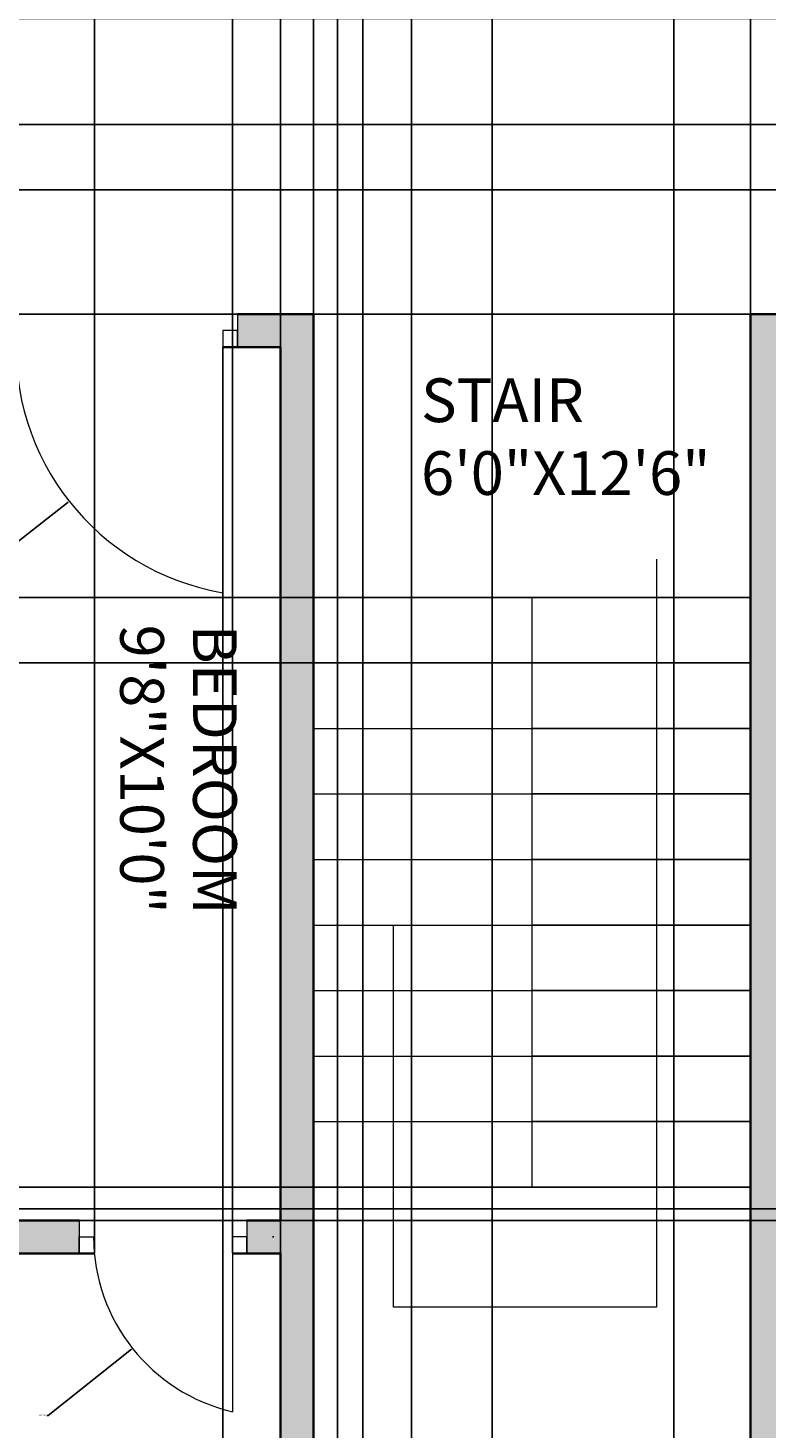
# Model space of a CAD drawing. Units: inches. Extents: x 2606 to 3027, y 1906 to 2463.
# Tile 3 of 10: x 2748 to 2850, y 2004 to 2196. Entities that reach past the tile are written whole.
import ezdxf

# ---------------------------------------------------------------- set-up
doc = ezdxf.new("R2010")
doc.units = ezdxf.units.IN
for name, color, linetype, lineweight in [('A-ANNO-DIMS', 2, 'Continuous', 18), ('A-AREA-IDEN', 7, 'Continuous', 18), ('A-DOOR', 3, 'Continuous', 18), ('A-FLOR-STRS', 7, 'Continuous', 18), ('A-WALL', 7, 'Continuous', 35)]:
    doc.layers.add(name, color=color, linetype=linetype, lineweight=lineweight)
doc.layers.add('A-WALL-PATT', color=251, linetype='Continuous', lineweight=13, true_color=0x636466)
doc.styles.get("Standard").update_dxf_attribs({"font": 'arial.ttf'})
doc.dimstyles.get("Standard").update_dxf_attribs({"dimtxt": 0.18, "dimasz": 0.18, "dimexe": 0.18, "dimexo": 0.0625, "dimgap": 0.09, "dimtad": 0, "dimtih": 1, "dimtoh": 1, "dimdec": 4, "dimzin": 0, "dimdsep": 46, "dimtxsty": 'Standard', "dimcen": 0.09, "dimadec": 0, "dimazin": 0, "dimtfac": 1, "dimtdec": 4, "dimtofl": 0, "dimtmove": 0, "dimatfit": 3, "dimfxl": 1, "dimtolj": 1, "dimtzin": 0, "dimarcsym": 0})

# ---------------------------------------------------------------- blocks, each defined once
blk = doc.blocks.new('*D34')
at = {"layer": 'A-ANNO-DIMS', "color": 0, "lineweight": -2, "transparency": 16777216}
for p, q in [((2787.56, 2118.27), (2787.56, 2433.99)), ((2787.74, 2433.81), (2817.34, 2433.81)), ((2847.38, 2433.81), (2817.78, 2433.81)), ((2847.56, 2118.27), (2847.56, 2433.99))]:
    blk.add_line(p, q, dxfattribs=at)
at = {"layer": 'A-ANNO-DIMS', "color": 0, "transparency": 16777216}
for points in [[(2787.74, 2433.84), (2787.74, 2433.78), (2787.56, 2433.81)], [(2847.38, 2433.84), (2847.38, 2433.78), (2847.56, 2433.81)]]:
    blk.add_solid(points, dxfattribs=at)
at = {"layer": 'Defpoints', "color": 0, "transparency": 16777216}
for p in [(2847.56, 2433.81), (2787.56, 2118.21), (2847.56, 2118.21)]:
    blk.add_point(p, dxfattribs=at)
at = {"layer": 'A-ANNO-DIMS', "color": 0, "transparency": 16777216, "insert": (2817.56, 2433.81), "char_height": 0.18, "attachment_point": 5}
blk.add_mtext('\\A1;60', dxfattribs=at)
blk = doc.blocks.new('*D35')
at = {"layer": 'A-ANNO-DIMS', "color": 0, "lineweight": -2, "transparency": 16777216}
for p, q in [((2801.04, 1993.17), (2801.04, 2433.99)), ((2801.22, 2433.81), (2818.82, 2433.81)), ((2836.86, 2433.81), (2819.26, 2433.81)), ((2837.04, 1993.17), (2837.04, 2433.99))]:
    blk.add_line(p, q, dxfattribs=at)
at = {"layer": 'A-ANNO-DIMS', "color": 0, "transparency": 16777216}
for points in [[(2801.22, 2433.84), (2801.22, 2433.78), (2801.04, 2433.81)], [(2836.86, 2433.84), (2836.86, 2433.78), (2837.04, 2433.81)]]:
    blk.add_solid(points, dxfattribs=at)
at = {"layer": 'Defpoints', "color": 0, "transparency": 16777216}
for p in [(2837.04, 2433.81), (2801.04, 1993.11), (2837.04, 1993.11)]:
    blk.add_point(p, dxfattribs=at)
at = {"layer": 'A-ANNO-DIMS', "color": 0, "transparency": 16777216, "insert": (2819.04, 2433.81), "char_height": 0.18, "attachment_point": 5}
blk.add_mtext('\\A1;36', dxfattribs=at)
blk = doc.blocks.new('*D36')
at = {"layer": 'A-ANNO-DIMS', "color": 0, "lineweight": -2, "transparency": 16777216}
for p, q in [((2787.56, 1993.17), (2787.56, 2433.99)), ((2787.74, 2433.81), (2793.85, 2433.81)), ((2800.86, 2433.81), (2794.76, 2433.81)), ((2801.04, 1993.17), (2801.04, 2433.99))]:
    blk.add_line(p, q, dxfattribs=at)
at = {"layer": 'A-ANNO-DIMS', "color": 0, "transparency": 16777216}
for points in [[(2787.74, 2433.84), (2787.74, 2433.78), (2787.56, 2433.81)], [(2800.86, 2433.84), (2800.86, 2433.78), (2801.04, 2433.81)]]:
    blk.add_solid(points, dxfattribs=at)
at = {"layer": 'Defpoints', "color": 0, "transparency": 16777216}
for p in [(2787.56, 2433.81), (2787.56, 1993.11), (2801.04, 1993.11)]:
    blk.add_point(p, dxfattribs=at)
at = {"layer": 'A-ANNO-DIMS', "color": 0, "transparency": 16777216, "insert": (2794.3, 2433.81), "char_height": 0.18, "attachment_point": 5}
blk.add_mtext('\\A1;13.478', dxfattribs=at)
blk = doc.blocks.new('*D38')
at = {"layer": 'A-ANNO-DIMS', "color": 0, "lineweight": -2, "transparency": 16777216}
for p, q in [((2783.06, 1993.17), (2783.06, 2433.99)), ((2783.24, 2433.81), (2785.05, 2433.81)), ((2787.38, 2433.81), (2785.57, 2433.81)), ((2787.56, 1993.17), (2787.56, 2433.99))]:
    blk.add_line(p, q, dxfattribs=at)
at = {"layer": 'A-ANNO-DIMS', "color": 0, "transparency": 16777216}
for points in [[(2783.24, 2433.84), (2783.24, 2433.78), (2783.06, 2433.81)], [(2787.38, 2433.84), (2787.38, 2433.78), (2787.56, 2433.81)]]:
    blk.add_solid(points, dxfattribs=at)
at = {"layer": 'Defpoints', "color": 0, "transparency": 16777216}
for p in [(2787.56, 2433.81), (2783.06, 1993.11), (2787.56, 1993.11)]:
    blk.add_point(p, dxfattribs=at)
at = {"layer": 'A-ANNO-DIMS', "color": 0, "transparency": 16777216, "insert": (2785.31, 2433.81), "char_height": 0.18, "attachment_point": 5}
blk.add_mtext('\\A1;4.5', dxfattribs=at)
blk = doc.blocks.new('*D39')
at = {"layer": 'A-ANNO-DIMS', "color": 0, "lineweight": -2, "transparency": 16777216}
for p, q in [((2847.5, 2118.21), (2634.68, 2118.21)), ((2634.86, 2118.03), (2634.86, 2113.89)), ((2634.86, 2109.39), (2634.86, 2113.53)), ((2847.5, 2109.21), (2634.68, 2109.21))]:
    blk.add_line(p, q, dxfattribs=at)
at = {"layer": 'A-ANNO-DIMS', "color": 0, "transparency": 16777216}
for points in [[(2634.83, 2118.03), (2634.89, 2118.03), (2634.86, 2118.21)], [(2634.83, 2109.39), (2634.89, 2109.39), (2634.86, 2109.21)]]:
    blk.add_solid(points, dxfattribs=at)
at = {"layer": 'Defpoints', "color": 0, "transparency": 16777216}
for p in [(2847.56, 2118.21), (2634.86, 2109.21), (2847.56, 2109.21)]:
    blk.add_point(p, dxfattribs=at)
at = {"layer": 'A-ANNO-DIMS', "color": 0, "transparency": 16777216, "insert": (2634.86, 2113.71), "char_height": 0.18, "attachment_point": 5}
blk.add_mtext('\\A1;9', dxfattribs=at)
blk = doc.blocks.new('*D40')
at = {"layer": 'A-ANNO-DIMS', "color": 0, "lineweight": -2, "transparency": 16777216}
for p, q in [((2847.5, 2037.21), (2634.68, 2037.21)), ((2634.86, 2037.03), (2634.86, 2015.34)), ((2634.86, 1993.29), (2634.86, 2014.98)), ((2847.5, 1993.11), (2634.68, 1993.11))]:
    blk.add_line(p, q, dxfattribs=at)
at = {"layer": 'A-ANNO-DIMS', "color": 0, "transparency": 16777216}
for points in [[(2634.83, 2037.03), (2634.89, 2037.03), (2634.86, 2037.21)], [(2634.83, 1993.29), (2634.89, 1993.29), (2634.86, 1993.11)]]:
    blk.add_solid(points, dxfattribs=at)
at = {"layer": 'Defpoints', "color": 0, "transparency": 16777216}
for p in [(2847.56, 2037.21), (2634.86, 1993.11), (2847.56, 1993.11)]:
    blk.add_point(p, dxfattribs=at)
at = {"layer": 'A-ANNO-DIMS', "color": 0, "transparency": 16777216, "insert": (2634.86, 2015.16), "char_height": 0.18, "attachment_point": 5}
blk.add_mtext('\\A1;44.1', dxfattribs=at)
blk = doc.blocks.new('*D41')
at = {"layer": 'A-ANNO-DIMS', "color": 0, "lineweight": -2, "transparency": 16777216}
for p, q in [((2787.63, 2157.11), (3000.44, 2157.11)), ((3000.26, 2156.93), (3000.26, 2075.29)), ((3000.26, 1993.29), (3000.26, 2074.93)), ((2787.63, 1993.11), (3000.44, 1993.11))]:
    blk.add_line(p, q, dxfattribs=at)
at = {"layer": 'A-ANNO-DIMS', "color": 0, "transparency": 16777216}
for points in [[(3000.23, 2156.93), (3000.29, 2156.93), (3000.26, 2157.11)], [(3000.23, 1993.29), (3000.29, 1993.29), (3000.26, 1993.11)]]:
    blk.add_solid(points, dxfattribs=at)
at = {"layer": 'Defpoints', "color": 0, "transparency": 16777216}
for p in [(2787.56, 2157.11), (2787.56, 1993.11), (3000.26, 1993.11)]:
    blk.add_point(p, dxfattribs=at)
at = {"layer": 'A-ANNO-DIMS', "color": 0, "transparency": 16777216, "insert": (3000.26, 2075.11), "char_height": 0.18, "attachment_point": 5}
blk.add_mtext('\\A1;164', dxfattribs=at)
blk = doc.blocks.new('*D43')
at = {"layer": 'A-ANNO-DIMS', "color": 0, "lineweight": -2, "transparency": 16777216}
for p, q in [((2794.34, 2257.55), (2794.34, 1965.23)), ((2812.09, 2257.55), (2812.09, 1965.23)), ((2794.52, 1965.41), (2802.76, 1965.41)), ((2811.91, 1965.41), (2803.67, 1965.41))]:
    blk.add_line(p, q, dxfattribs=at)
at = {"layer": 'A-ANNO-DIMS', "color": 0, "transparency": 16777216}
for points in [[(2794.52, 1965.44), (2794.52, 1965.38), (2794.34, 1965.41)], [(2811.91, 1965.44), (2811.91, 1965.38), (2812.09, 1965.41)]]:
    blk.add_solid(points, dxfattribs=at)
at = {"layer": 'Defpoints', "color": 0, "transparency": 16777216}
for p in [(2794.34, 2257.61), (2812.09, 2257.61), (2812.09, 1965.41)]:
    blk.add_point(p, dxfattribs=at)
at = {"layer": 'A-ANNO-DIMS', "color": 0, "transparency": 16777216, "insert": (2803.22, 1965.41), "char_height": 0.18, "attachment_point": 5}
blk.add_mtext('\\A1;17.756', dxfattribs=at)
blk = doc.blocks.new('*D45')
at = {"layer": 'A-ANNO-DIMS', "color": 0, "lineweight": -2, "transparency": 16777216}
for p, q in [((2746.75, 2152.55), (2746.75, 1965.23)), ((2775.13, 2152.55), (2775.13, 1965.23)), ((2746.93, 1965.41), (2760.47, 1965.41)), ((2774.95, 1965.41), (2761.4, 1965.41))]:
    blk.add_line(p, q, dxfattribs=at)
at = {"layer": 'A-ANNO-DIMS', "color": 0, "transparency": 16777216}
for points in [[(2746.93, 1965.44), (2746.93, 1965.38), (2746.75, 1965.41)], [(2774.95, 1965.44), (2774.95, 1965.38), (2775.13, 1965.41)]]:
    blk.add_solid(points, dxfattribs=at)
at = {"layer": 'Defpoints', "color": 0, "transparency": 16777216}
for p in [(2746.75, 2152.61), (2775.13, 2152.61), (2775.13, 1965.41)]:
    blk.add_point(p, dxfattribs=at)
at = {"layer": 'A-ANNO-DIMS', "color": 0, "transparency": 16777216, "insert": (2760.94, 1965.41), "char_height": 0.18, "attachment_point": 5}
blk.add_mtext('\\A1;28.384', dxfattribs=at)
blk = doc.blocks.new('*D47')
at = {"layer": 'A-ANNO-DIMS', "color": 0, "lineweight": -2, "transparency": 16777216}
for p, q in [((2757.51, 2028.17), (2757.51, 2433.99)), ((2757.69, 2433.81), (2766.59, 2433.81)), ((2776.27, 2433.81), (2767.36, 2433.81)), ((2776.45, 2028.17), (2776.45, 2433.99))]:
    blk.add_line(p, q, dxfattribs=at)
at = {"layer": 'A-ANNO-DIMS', "color": 0, "transparency": 16777216}
for points in [[(2757.69, 2433.84), (2757.69, 2433.78), (2757.51, 2433.81)], [(2776.27, 2433.84), (2776.27, 2433.78), (2776.45, 2433.81)]]:
    blk.add_solid(points, dxfattribs=at)
at = {"layer": 'Defpoints', "color": 0, "transparency": 16777216}
for p in [(2776.45, 2433.81), (2757.51, 2028.11), (2776.45, 2028.11)]:
    blk.add_point(p, dxfattribs=at)
at = {"layer": 'A-ANNO-DIMS', "color": 0, "transparency": 16777216, "insert": (2766.98, 2433.81), "char_height": 0.18, "attachment_point": 5}
blk.add_mtext('\\A1;18.94', dxfattribs=at)
blk = doc.blocks.new('*D52')
at = {"layer": 'A-ANNO-DIMS', "color": 0, "lineweight": -2, "transparency": 16777216}
for p, q in [((2787.56, 2257.55), (2787.56, 1965.23)), ((2794.34, 2257.55), (2794.34, 1965.23)), ((2787.74, 1965.41), (2790.56, 1965.41)), ((2794.16, 1965.41), (2791.34, 1965.41))]:
    blk.add_line(p, q, dxfattribs=at)
at = {"layer": 'A-ANNO-DIMS', "color": 0, "transparency": 16777216}
for points in [[(2787.74, 1965.44), (2787.74, 1965.38), (2787.56, 1965.41)], [(2794.16, 1965.44), (2794.16, 1965.38), (2794.34, 1965.41)]]:
    blk.add_solid(points, dxfattribs=at)
at = {"layer": 'Defpoints', "color": 0, "transparency": 16777216}
for p in [(2787.56, 2257.61), (2794.34, 2257.61), (2794.34, 1965.41)]:
    blk.add_point(p, dxfattribs=at)
at = {"layer": 'A-ANNO-DIMS', "color": 0, "transparency": 16777216, "insert": (2790.95, 1965.41), "char_height": 0.18, "attachment_point": 5}
blk.add_mtext('\\A1;6.776', dxfattribs=at)
blk = doc.blocks.new('*D54')
at = {"layer": 'A-ANNO-DIMS', "color": 0, "lineweight": -2, "transparency": 16777216}
for p, q in [((2775.13, 2152.55), (2775.13, 1965.23)), ((2783.06, 2152.55), (2783.06, 1965.23)), ((2775.31, 1965.41), (2778.7, 1965.41)), ((2782.88, 1965.41), (2779.49, 1965.41))]:
    blk.add_line(p, q, dxfattribs=at)
at = {"layer": 'A-ANNO-DIMS', "color": 0, "transparency": 16777216}
for points in [[(2775.31, 1965.44), (2775.31, 1965.38), (2775.13, 1965.41)], [(2782.88, 1965.44), (2782.88, 1965.38), (2783.06, 1965.41)]]:
    blk.add_solid(points, dxfattribs=at)
at = {"layer": 'Defpoints', "color": 0, "transparency": 16777216}
for p in [(2775.13, 2152.61), (2783.06, 2152.61), (2783.06, 1965.41)]:
    blk.add_point(p, dxfattribs=at)
at = {"layer": 'A-ANNO-DIMS', "color": 0, "transparency": 16777216, "insert": (2779.1, 1965.41), "char_height": 0.18, "attachment_point": 5}
blk.add_mtext('\\A1;7.933', dxfattribs=at)
blk = doc.blocks.new('*D56')
at = {"layer": 'A-ANNO-DIMS', "color": 0, "lineweight": -2, "transparency": 16777216}
for p, q in [((2776.45, 2028.17), (2776.45, 2433.99)), ((2776.63, 2433.81), (2779.36, 2433.81)), ((2782.88, 2433.81), (2780.15, 2433.81)), ((2783.06, 2032.67), (2783.06, 2433.99))]:
    blk.add_line(p, q, dxfattribs=at)
at = {"layer": 'A-ANNO-DIMS', "color": 0, "transparency": 16777216}
for points in [[(2776.63, 2433.84), (2776.63, 2433.78), (2776.45, 2433.81)], [(2782.88, 2433.84), (2782.88, 2433.78), (2783.06, 2433.81)]]:
    blk.add_solid(points, dxfattribs=at)
at = {"layer": 'Defpoints', "color": 0, "transparency": 16777216}
for p in [(2783.06, 2433.81), (2783.06, 2032.61), (2776.45, 2028.11)]:
    blk.add_point(p, dxfattribs=at)
at = {"layer": 'A-ANNO-DIMS', "color": 0, "transparency": 16777216, "insert": (2779.76, 2433.81), "char_height": 0.18, "attachment_point": 5}
blk.add_mtext('\\A1;6.615', dxfattribs=at)
blk = doc.blocks.new('*D61')
at = {"layer": 'A-ANNO-DIMS', "color": 0, "lineweight": -2, "transparency": 16777216}
for p, q in [((2696.29, 2197.72), (3000.44, 2197.72)), ((3000.26, 2197.54), (3000.26, 2190.63)), ((3000.26, 2183.36), (3000.26, 2190.27)), ((2696.84, 2183.18), (3000.44, 2183.18))]:
    blk.add_line(p, q, dxfattribs=at)
at = {"layer": 'A-ANNO-DIMS', "color": 0, "transparency": 16777216}
for points in [[(3000.23, 2197.54), (3000.29, 2197.54), (3000.26, 2197.72)], [(3000.23, 2183.36), (3000.29, 2183.36), (3000.26, 2183.18)]]:
    blk.add_solid(points, dxfattribs=at)
at = {"layer": 'Defpoints', "color": 0, "transparency": 16777216}
for p in [(2696.23, 2197.72), (3000.26, 2197.72), (2696.78, 2183.18)]:
    blk.add_point(p, dxfattribs=at)
at = {"layer": 'A-ANNO-DIMS', "color": 0, "transparency": 16777216, "insert": (3000.26, 2190.45), "char_height": 0.18, "attachment_point": 5}
blk.add_mtext('\\A1;14.545', dxfattribs=at)
blk = doc.blocks.new('*D68')
at = {"layer": 'A-ANNO-DIMS', "color": 0, "lineweight": -2, "transparency": 16777216}
for p, q in [((2897, 2215.13), (2634.68, 2215.13)), ((2634.86, 2214.95), (2634.86, 2194.85)), ((2634.86, 2174.38), (2634.86, 2194.48)), ((2897, 2174.2), (2634.68, 2174.2))]:
    blk.add_line(p, q, dxfattribs=at)
at = {"layer": 'A-ANNO-DIMS', "color": 0, "transparency": 16777216}
for points in [[(2634.83, 2214.95), (2634.89, 2214.95), (2634.86, 2215.13)], [(2634.83, 2174.38), (2634.89, 2174.38), (2634.86, 2174.2)]]:
    blk.add_solid(points, dxfattribs=at)
at = {"layer": 'Defpoints', "color": 0, "transparency": 16777216}
for p in [(2897.06, 2215.13), (2634.86, 2174.2), (2897.06, 2174.2)]:
    blk.add_point(p, dxfattribs=at)
at = {"layer": 'A-ANNO-DIMS', "color": 0, "transparency": 16777216, "insert": (2634.86, 2194.66), "char_height": 0.18, "attachment_point": 5}
blk.add_mtext('\\A1;40.94', dxfattribs=at)
blk = doc.blocks.new('*D69')
at = {"layer": 'A-ANNO-DIMS', "color": 0, "lineweight": -2, "transparency": 16777216}
for p, q in [((2897, 2174.2), (2634.68, 2174.2)), ((2634.86, 2174.02), (2634.86, 2165.84)), ((2634.86, 2157.29), (2634.86, 2165.47)), ((2897, 2157.11), (2634.68, 2157.11))]:
    blk.add_line(p, q, dxfattribs=at)
at = {"layer": 'A-ANNO-DIMS', "color": 0, "transparency": 16777216}
for points in [[(2634.83, 2174.02), (2634.89, 2174.02), (2634.86, 2174.2)], [(2634.83, 2157.29), (2634.89, 2157.29), (2634.86, 2157.11)]]:
    blk.add_solid(points, dxfattribs=at)
at = {"layer": 'Defpoints', "color": 0, "transparency": 16777216}
for p in [(2897.06, 2174.2), (2634.86, 2157.11), (2897.06, 2157.11)]:
    blk.add_point(p, dxfattribs=at)
at = {"layer": 'A-ANNO-DIMS', "color": 0, "transparency": 16777216, "insert": (2634.86, 2165.65), "char_height": 0.18, "attachment_point": 5}
blk.add_mtext('\\A1;17.087', dxfattribs=at)
blk = doc.blocks.new('*D76')
at = {"layer": 'A-ANNO-DIMS', "color": 0, "lineweight": -2, "transparency": 16777216}
for p, q in [((2738.62, 2035.66), (2738.62, 2433.99)), ((2738.8, 2433.81), (2760.37, 2433.81)), ((2782.88, 2433.81), (2761.31, 2433.81)), ((2783.06, 2032.67), (2783.06, 2433.99))]:
    blk.add_line(p, q, dxfattribs=at)
at = {"layer": 'A-ANNO-DIMS', "color": 0, "transparency": 16777216}
for points in [[(2738.8, 2433.84), (2738.8, 2433.78), (2738.62, 2433.81)], [(2782.88, 2433.84), (2782.88, 2433.78), (2783.06, 2433.81)]]:
    blk.add_solid(points, dxfattribs=at)
at = {"layer": 'Defpoints', "color": 0, "transparency": 16777216}
for p in [(2783.06, 2433.81), (2738.62, 2035.6), (2783.06, 2032.61)]:
    blk.add_point(p, dxfattribs=at)
at = {"layer": 'A-ANNO-DIMS', "color": 0, "transparency": 16777216, "insert": (2760.84, 2433.81), "char_height": 0.18, "attachment_point": 5}
blk.add_mtext('\\A1;44.445', dxfattribs=at)
blk = doc.blocks.new('*D81')
at = {"layer": 'A-ANNO-DIMS', "color": 0, "lineweight": -2, "transparency": 16777216}
for p, q in [((2961.6, 2034.23), (2634.68, 2034.23)), ((2634.86, 2034.05), (2634.86, 2033.6)), ((2634.86, 2032.79), (2634.86, 2033.24)), ((2950.83, 2032.61), (2634.68, 2032.61))]:
    blk.add_line(p, q, dxfattribs=at)
at = {"layer": 'A-ANNO-DIMS', "color": 0, "transparency": 16777216}
for points in [[(2634.83, 2034.05), (2634.89, 2034.05), (2634.86, 2034.23)], [(2634.83, 2032.79), (2634.89, 2032.79), (2634.86, 2032.61)]]:
    blk.add_solid(points, dxfattribs=at)
at = {"layer": 'Defpoints', "color": 0, "transparency": 16777216}
for p in [(2961.66, 2034.23), (2634.86, 2032.61), (2950.89, 2032.61)]:
    blk.add_point(p, dxfattribs=at)
at = {"layer": 'A-ANNO-DIMS', "color": 0, "transparency": 16777216, "insert": (2634.86, 2033.42), "char_height": 0.18, "attachment_point": 5}
blk.add_mtext('\\A1;1.62', dxfattribs=at)
blk = doc.blocks.new('*D83')
at = {"layer": 'A-ANNO-DIMS', "color": 0, "lineweight": -2, "transparency": 16777216}
for p, q in [((2787.56, 2327.05), (2787.56, 1965.23)), ((2790.85, 2327.05), (2790.85, 1965.23)), ((2787.74, 1965.41), (2788.88, 1965.41)), ((2790.67, 1965.41), (2789.53, 1965.41))]:
    blk.add_line(p, q, dxfattribs=at)
at = {"layer": 'A-ANNO-DIMS', "color": 0, "transparency": 16777216}
for points in [[(2787.74, 1965.44), (2787.74, 1965.38), (2787.56, 1965.41)], [(2790.67, 1965.44), (2790.67, 1965.38), (2790.85, 1965.41)]]:
    blk.add_solid(points, dxfattribs=at)
at = {"layer": 'Defpoints', "color": 0, "transparency": 16777216}
for p in [(2787.56, 2327.11), (2790.85, 2327.11), (2790.85, 1965.41)]:
    blk.add_point(p, dxfattribs=at)
at = {"layer": 'A-ANNO-DIMS', "color": 0, "transparency": 16777216, "insert": (2789.21, 1965.41), "char_height": 0.18, "attachment_point": 5}
blk.add_mtext('\\A1;3.29', dxfattribs=at)
blk = doc.blocks.new('*D86')
at = {"layer": 'A-ANNO-DIMS', "color": 0, "lineweight": -2, "transparency": 16777216}
for p, q in [((2780.83, 2152.54), (2781.01, 2152.54)), ((2780.92, 2152.45), (2780.92, 2152.63)), ((2737.93, 2118.74), (2753.91, 2131.31)), ((2737.75, 2118.74), (2737.93, 2118.74))]:
    blk.add_line(p, q, dxfattribs=at)
at = {"layer": 'A-ANNO-DIMS', "color": 0, "transparency": 16777216}
blk.add_solid([(2753.9, 2131.33), (2753.93, 2131.28), (2754.06, 2131.42)], dxfattribs=at)
at = {"layer": 'Defpoints', "color": 0, "transparency": 16777216}
for p in [(2780.92, 2152.54), (2754.06, 2131.42)]:
    blk.add_point(p, dxfattribs=at)
at = {"layer": 'A-ANNO-DIMS', "color": 0, "transparency": 16777216, "insert": (2737.27, 2118.74), "char_height": 0.18, "attachment_point": 5}
blk.add_mtext('\\A1;R34.18', dxfattribs=at)
blk = doc.blocks.new('*D88')
at = {"layer": 'A-ANNO-DIMS', "color": 0, "lineweight": -2, "transparency": 16777216}
for p, q in [((2781.96, 2030.36), (2782.14, 2030.36)), ((2782.05, 2030.27), (2782.05, 2030.45)), ((2751.16, 2005.85), (2762.6, 2014.93)), ((2750.98, 2005.85), (2751.16, 2005.85))]:
    blk.add_line(p, q, dxfattribs=at)
at = {"layer": 'A-ANNO-DIMS', "color": 0, "transparency": 16777216}
blk.add_solid([(2762.59, 2014.95), (2762.62, 2014.91), (2762.75, 2015.04)], dxfattribs=at)
at = {"layer": 'Defpoints', "color": 0, "transparency": 16777216}
for p in [(2782.05, 2030.36), (2762.75, 2015.04)]:
    blk.add_point(p, dxfattribs=at)
at = {"layer": 'A-ANNO-DIMS', "color": 0, "transparency": 16777216, "insert": (2750.43, 2005.85), "char_height": 0.18, "attachment_point": 5}
blk.add_mtext('\\A1;R24.646', dxfattribs=at)

msp = doc.modelspace()

# ---------------------------------------------------------------- hatches: boundary and pattern name
at = {"layer": 'A-WALL-PATT'}
h = msp.add_hatch(color=256, dxfattribs=at)
h.dxf.hatch_style = 1
h.paths.add_polyline_path([(2667.063, 2401.6097), (2691.9697, 2401.6097), (2691.9697, 2406.1097), (2691.9697, 2410.6097), (2658.063, 2410.6097), (2658.063, 2238.7051), (2667.063, 2238.7051)])
h.paths.add_polyline_path([(2804.9965, 2406.1097), (2804.9965, 2410.6097), (2751.9697, 2410.6097), (2751.9697, 2401.6097), (2783.063, 2401.6097), (2783.063, 2257.6097), (2778.6739, 2257.6097), (2778.6739, 2253.1097), (2792.3386, 2253.1097), (2792.3386, 2255.3597), (2792.3386, 2257.6097), (2787.563, 2257.6097), (2787.563, 2327.1097), (2847.563, 2327.1097), (2847.563, 2331.6097), (2787.563, 2331.6097), (2787.563, 2401.6097), (2804.9965, 2401.6097)])
h.paths.add_polyline_path([(2889.6183, 2406.1097), (2889.6183, 2410.6097), (2828.9965, 2410.6097), (2828.9965, 2401.6097), (2831.8174, 2401.6097), (2847.563, 2401.6097), (2847.563, 2357.8311), (2849.813, 2357.8311), (2852.063, 2357.8311), (2852.063, 2401.6097), (2889.6183, 2401.6097)])
h.paths.add_polyline_path([(2977.063, 2410.6097), (2949.6183, 2410.6097), (2949.6183, 2401.6097), (2968.063, 2401.6097), (2968.063, 2157.1097), (2897.063, 2157.1097), (2897.063, 2174.1966), (2892.563, 2174.1966), (2892.563, 2157.1097), (2886.8122, 2157.1097), (2886.8122, 2152.6097), (2968.063, 2152.6097), (2968.063, 2032.6097), (2950.8911, 2032.6097), (2950.8911, 2028.1097), (2968.063, 2028.1097), (2968.063, 1993.1097), (2852.063, 1993.1097), (2852.063, 2028.1097), (2856.0743, 2028.1097), (2856.0743, 2030.3597), (2856.0743, 2032.6097), (2852.063, 2032.6097), (2852.063, 2152.6097), (2857.369, 2152.6097), (2857.369, 2154.8597), (2857.369, 2157.1097), (2847.563, 2157.1097), (2847.563, 2152.6097), (2847.563, 1993.1097), (2837.0415, 1993.1097), (2837.0415, 1988.6097), (2977.063, 1988.6097)])
h.paths.add_polyline_path([(2968.063, 2257.6097), (2886.9679, 2257.6097), (2886.9679, 2253.1097), (2892.563, 2253.1097), (2892.563, 2215.1332), (2897.063, 2215.1332), (2897.063, 2253.1097), (2968.063, 2253.1097)], flags=17)
h.paths.add_polyline_path([(2856.057, 2255.3597), (2856.057, 2257.6097), (2852.063, 2257.6097), (2852.063, 2336.7476), (2849.813, 2336.7476), (2847.563, 2336.7476), (2847.563, 2331.6097), (2847.563, 2327.1097), (2847.563, 2257.6097), (2813.482, 2257.6097), (2813.482, 2253.1097), (2856.057, 2253.1097)])
h.paths.add_polyline_path([(2748.8874, 2255.3597), (2748.8874, 2257.6097), (2667.063, 2257.6097), (2667.063, 2253.1097), (2748.8874, 2253.1097)])
h.paths.add_polyline_path([(2667.063, 2152.6097), (2744.8238, 2152.6097), (2744.8238, 2154.8597), (2744.8238, 2157.1097), (2667.063, 2157.1097), (2667.063, 2178.7051), (2658.063, 2178.7051), (2658.063, 1988.6097), (2801.0415, 1988.6097), (2801.0415, 1990.8597), (2801.0415, 1993.1097), (2787.563, 1993.1097), (2787.563, 2157.1097), (2777.1295, 2157.1097), (2777.1295, 2152.6097), (2783.063, 2152.6097), (2783.063, 2032.6097), (2778.4484, 2032.6097), (2778.4484, 2028.1097), (2783.063, 2028.1097), (2783.063, 1993.1097), (2667.063, 1993.1097), (2667.063, 2028.1097), (2680.1652, 2028.1097), (2680.1652, 2030.3597), (2680.1652, 2032.6097), (2667.063, 2032.6097)])
h.paths.add_polyline_path([(2755.4074, 2032.6097), (2728.1652, 2032.6097), (2728.1652, 2028.1097), (2755.4074, 2028.1097), (2755.4074, 2030.3597)], flags=17)
h.paths.add_polyline_path([(2902.8911, 2030.3597), (2902.8911, 2032.6097), (2877.6885, 2032.6097), (2877.6885, 2028.1097), (2902.8911, 2028.1097)], flags=17)
h.paths.add_polyline_path([(2810.2211, 2267.221), (2851.2716, 2267.221), (2851.2716, 2289.6098), (2810.2211, 2289.6098)], flags=9)

# ---------------------------------------------------------------- linework, layer by layer
at = {"layer": 'A-DOOR'}
for p, q in [((2777.1295, 2157.1097), (2777.1295, 2152.6097)), ((2777.1295, 2154.8597), (2775.1295, 2154.8597)), ((2775.1295, 2154.8597), (2775.1295, 2118.8597)), ((2777.1295, 2152.6097), (2777.1295, 2154.8597)), ((2755.4074, 2032.6097), (2755.4074, 2028.1097)), ((2778.4484, 2032.6097), (2778.4484, 2032.6097)), ((2778.4484, 2032.6097), (2778.4484, 2028.1097)), ((2755.4074, 2028.1097), (2755.4074, 2030.3597)), ((2755.4074, 2030.3597), (2757.4074, 2030.3597)), ((2778.4484, 2030.3597), (2776.4484, 2030.3597)), ((2776.4484, 2030.3597), (2776.4484, 2006.3597)), ((2778.4484, 2028.1097), (2778.4484, 2030.3597))]:
    msp.add_line(p, q, dxfattribs=at)
for centre, radius, start, end in [((2780.9223, 2152.5424), 34.1772, 176.112165, 260.241721), ((2782.0531, 2030.3597), 24.6457, 180, 256.855288)]:
    msp.add_arc(centre, radius, start, end, dxfattribs=at)
at = {"layer": 'A-FLOR-STRS'}
for p, q in [((2834.6516, 2123.4613), (2834.6516, 2020.7113)), ((2787.563, 2118.2123), (2847.563, 2118.2123)), ((2847.563, 2118.2123), (2817.563, 2118.2123)), ((2817.563, 2118.2123), (2817.563, 2037.2123)), ((2787.563, 2109.2123), (2847.563, 2109.2123)), ((2847.563, 2109.2123), (2817.563, 2109.2123)), ((2787.563, 2100.2123), (2847.563, 2100.2123)), ((2847.563, 2100.2123), (2817.563, 2100.2123)), ((2787.563, 2091.2123), (2847.563, 2091.2123)), ((2847.563, 2091.2123), (2817.563, 2091.2123)), ((2787.563, 2082.2123), (2847.563, 2082.2123)), ((2847.563, 2082.2123), (2817.563, 2082.2123)), ((2787.563, 2073.2123), (2847.563, 2073.2123)), ((2798.5609, 2020.7113), (2798.5609, 2073.2123)), ((2847.563, 2073.2123), (2817.563, 2073.2123)), ((2787.563, 2064.2123), (2847.563, 2064.2123)), ((2847.563, 2064.2123), (2817.563, 2064.2123)), ((2787.563, 2055.2123), (2847.563, 2055.2123)), ((2847.563, 2055.2123), (2817.563, 2055.2123)), ((2787.563, 2046.2123), (2847.563, 2046.2123)), ((2847.563, 2046.2123), (2817.563, 2046.2123)), ((2787.563, 2037.2123), (2847.563, 2037.2123)), ((2847.563, 2037.2123), (2817.563, 2037.2123)), ((2834.6516, 2020.7113), (2798.5609, 2020.7113))]:
    msp.add_line(p, q, dxfattribs=at)
at = {"layer": 'A-WALL'}
for p, q in [((2787.563, 2157.1097), (2777.1295, 2157.1097)), ((2777.1295, 2157.1097), (2787.563, 2157.1097)), ((2787.563, 2157.1097), (2787.563, 1993.1097)), ((2847.563, 2152.6097), (2847.563, 2157.1097)), ((2847.563, 2157.1097), (2857.369, 2157.1097)), ((2847.563, 2157.1097), (2857.369, 2157.1097)), ((2775.1295, 2152.6097), (2783.063, 2152.6097)), ((2783.063, 2152.6097), (2783.063, 2032.6097)), ((2847.563, 2152.6097), (2847.563, 1993.1097)), ((2667.063, 2032.6097), (2755.4074, 2032.6097)), ((2778.4484, 2032.6097), (2783.063, 2032.6097)), ((2667.063, 2028.1097), (2757.5103, 2028.1097)), ((2776.4484, 2028.1097), (2783.063, 2028.1097)), ((2783.063, 2028.1097), (2783.063, 1993.1097))]:
    msp.add_line(p, q, dxfattribs=at)

# ---------------------------------------------------------------- texts
at = {"layer": 'A-AREA-IDEN', "insert": (2802.3425, 2148.2933), "char_height": 6, "attachment_point": 1}
msp.add_mtext_dynamic_manual_height_columns('STAIR\\P6\'0"X12\'6"', width=27.625327, gutter_width=12.5, heights=[0], dxfattribs=at)
at = {"layer": 'A-AREA-IDEN', "insert": (2777.0556, 2114.4746), "char_height": 6, "attachment_point": 1, "rotation": 270}
msp.add_mtext_dynamic_manual_height_columns('BEDROOM\\P9\'8"X10\'0"', width=91.526124, gutter_width=12.5, heights=[0], dxfattribs=at)

# ---------------------------------------------------------------- dimensions: what is measured, and where the dimension line sits
at = {"layer": 'A-ANNO-DIMS'}
for base, p1, p2, override, picture, middle in [((2783.063, 2433.8097), (2738.6178, 2035.5977), (2783.063, 2032.6097), {"dimdec": 3, "dimlfac": 1, "dimrnd": 0, "dimzin": 0, "dimdsep": 46, "dimlunit": 2}, '*D76', (2760.8404, 2433.8097)), ((2776.4484, 2433.8097), (2757.5103, 2028.1097), (2776.4484, 2028.1097), {"dimdec": 2, "dimlfac": 1, "dimrnd": 0, "dimzin": 0, "dimdsep": 46, "dimlunit": 2}, '*D47', (2766.9794, 2433.8097)), ((2783.063, 2433.8097), (2776.4484, 2028.1097), (2783.063, 2032.6097), {"dimdec": 3, "dimlfac": 1, "dimrnd": 0, "dimzin": 0, "dimdsep": 46, "dimlunit": 2}, '*D56', (2779.7557, 2433.8097)), ((2787.563, 2433.8097), (2783.063, 1993.1097), (2787.563, 1993.1097), {"dimdec": 1, "dimlfac": 1, "dimrnd": 0, "dimzin": 0, "dimdsep": 46, "dimlunit": 2}, '*D38', (2785.313, 2433.8097)), ((2847.563, 2433.8097), (2787.563, 2118.2123), (2847.563, 2118.2123), {"dimdec": 0, "dimlfac": 1, "dimrnd": 0, "dimzin": 0, "dimdsep": 46, "dimlunit": 2}, '*D34', (2817.563, 2433.8097)), ((2787.56299, 2433.8097), (2801.04146, 1993.1097), (2787.56299, 1993.1097), {"dimdec": 3, "dimlfac": 1, "dimrnd": 0, "dimzin": 0, "dimdsep": 46, "dimlunit": 2}, '*D36', (2794.30223, 2433.8097)), ((2837.0415, 2433.8097), (2801.0415, 1993.1097), (2837.0415, 1993.1097), {"dimdec": 0, "dimlfac": 1, "dimrnd": 0, "dimzin": 0, "dimdsep": 46, "dimlunit": 2}, '*D35', (2819.0415, 2433.8097)), ((2790.8496, 1965.4097), (2787.563, 2327.1097), (2790.8496, 2327.1097), {"dimdec": 2, "dimlfac": 1, "dimrnd": 0, "dimzin": 0, "dimdsep": 46, "dimlunit": 2}, '*D83', (2789.2063, 1965.4097)), ((2794.3386, 1965.4097), (2787.563, 2257.6097), (2794.3386, 2257.6097), {"dimdec": 3, "dimlfac": 1, "dimrnd": 0, "dimzin": 0, "dimdsep": 46, "dimlunit": 2}, '*D52', (2790.9508, 1965.4097)), ((2812.0947, 1965.4097), (2794.3386, 2257.6097), (2812.0947, 2257.6097), {"dimdec": 3, "dimlfac": 1, "dimrnd": 0, "dimzin": 0, "dimdsep": 46, "dimlunit": 2}, '*D43', (2803.2167, 1965.4097)), ((2775.1295, 1965.4097), (2746.7452, 2152.6097), (2775.1295, 2152.6097), {"dimdec": 3, "dimlfac": 1, "dimrnd": 0, "dimzin": 0, "dimdsep": 46, "dimlunit": 2}, '*D45', (2760.9374, 1965.4097)), ((2783.06299, 1965.4097), (2775.12954, 2152.6097), (2783.06299, 2152.6097), {"dimdec": 3, "dimlfac": 1, "dimrnd": 0, "dimzin": 0, "dimdsep": 46, "dimlunit": 2}, '*D54', (2779.09627, 1965.4097))]:
    dim = msp.add_linear_dim(base=base, p1=p1, p2=p2, dimstyle='Standard', override=override, dxfattribs=at)
    dim.commit()
    dim.dimension.update_dxf_attribs({"geometry": picture, "text_midpoint": middle})
for base, p1, p2, override, picture, middle in [((2634.863, 2174.1966), (2897.063, 2215.1332), (2897.063, 2174.1966), {"dimdec": 2, "dimlfac": 1, "dimrnd": 0, "dimzin": 0, "dimdsep": 46, "dimlunit": 2}, '*D68', (2634.863, 2194.6649)), ((3000.263, 2197.7249), (2696.782, 2183.1802), (2696.232, 2197.7249), {"dimdec": 3, "dimlfac": 1, "dimrnd": 0, "dimzin": 0, "dimdsep": 46, "dimlunit": 2}, '*D61', (3000.263, 2190.4526)), ((2634.863, 2157.1097), (2897.063, 2174.1966), (2897.063, 2157.1097), {"dimdec": 3, "dimlfac": 1, "dimrnd": 0, "dimzin": 0, "dimdsep": 46, "dimlunit": 2}, '*D69', (2634.863, 2165.6532)), ((3000.263, 1993.1097), (2787.563, 2157.1097), (2787.563, 1993.1097), {"dimdec": 0, "dimlfac": 1, "dimrnd": 0, "dimzin": 0, "dimdsep": 46, "dimlunit": 2}, '*D41', (3000.263, 2075.1097)), ((2634.863, 2109.2123), (2847.563, 2118.2123), (2847.563, 2109.2123), {"dimdec": 0, "dimlfac": 1, "dimrnd": 0, "dimzin": 0, "dimdsep": 46, "dimlunit": 2}, '*D39', (2634.863, 2113.7123)), ((2634.863, 1993.1097), (2847.563, 2037.2123), (2847.563, 1993.1097), {"dimdec": 1, "dimlfac": 1, "dimrnd": 0, "dimzin": 0, "dimdsep": 46, "dimlunit": 2}, '*D40', (2634.863, 2015.161)), ((2634.863, 2032.6097), (2961.6611, 2034.2301), (2950.8911, 2032.6097), {"dimdec": 2, "dimlfac": 1, "dimrnd": 0, "dimzin": 0, "dimdsep": 46, "dimlunit": 2}, '*D81', (2634.863, 2033.4199))]:
    dim = msp.add_linear_dim(base=base, p1=p1, p2=p2, angle=90, dimstyle='Standard', override=override, dxfattribs=at)
    dim.commit()
    dim.dimension.update_dxf_attribs({"geometry": picture, "text_midpoint": middle})
for center, mpoint, override, picture, middle in [((2780.9223, 2152.5424), (2754.0551, 2131.4181), {"dimdec": 2, "dimlfac": 1, "dimrnd": 0, "dimzin": 0, "dimdsep": 46, "dimlunit": 2}, '*D86', (2737.2748, 2118.7436)), ((2782.0531, 2030.3597), (2762.7457, 2015.0418), {"dimdec": 3, "dimlfac": 1, "dimrnd": 0, "dimzin": 0, "dimdsep": 46, "dimlunit": 2}, '*D88', (2750.4316, 2005.8511))]:
    dim = msp.add_radius_dim(center=center, mpoint=mpoint, dimstyle='Standard', override=override, dxfattribs=at)
    dim.commit()
    dim.dimension.update_dxf_attribs({"geometry": picture, "text_midpoint": middle, "dimtype": 164})

doc.saveas('drawing.dxf')
